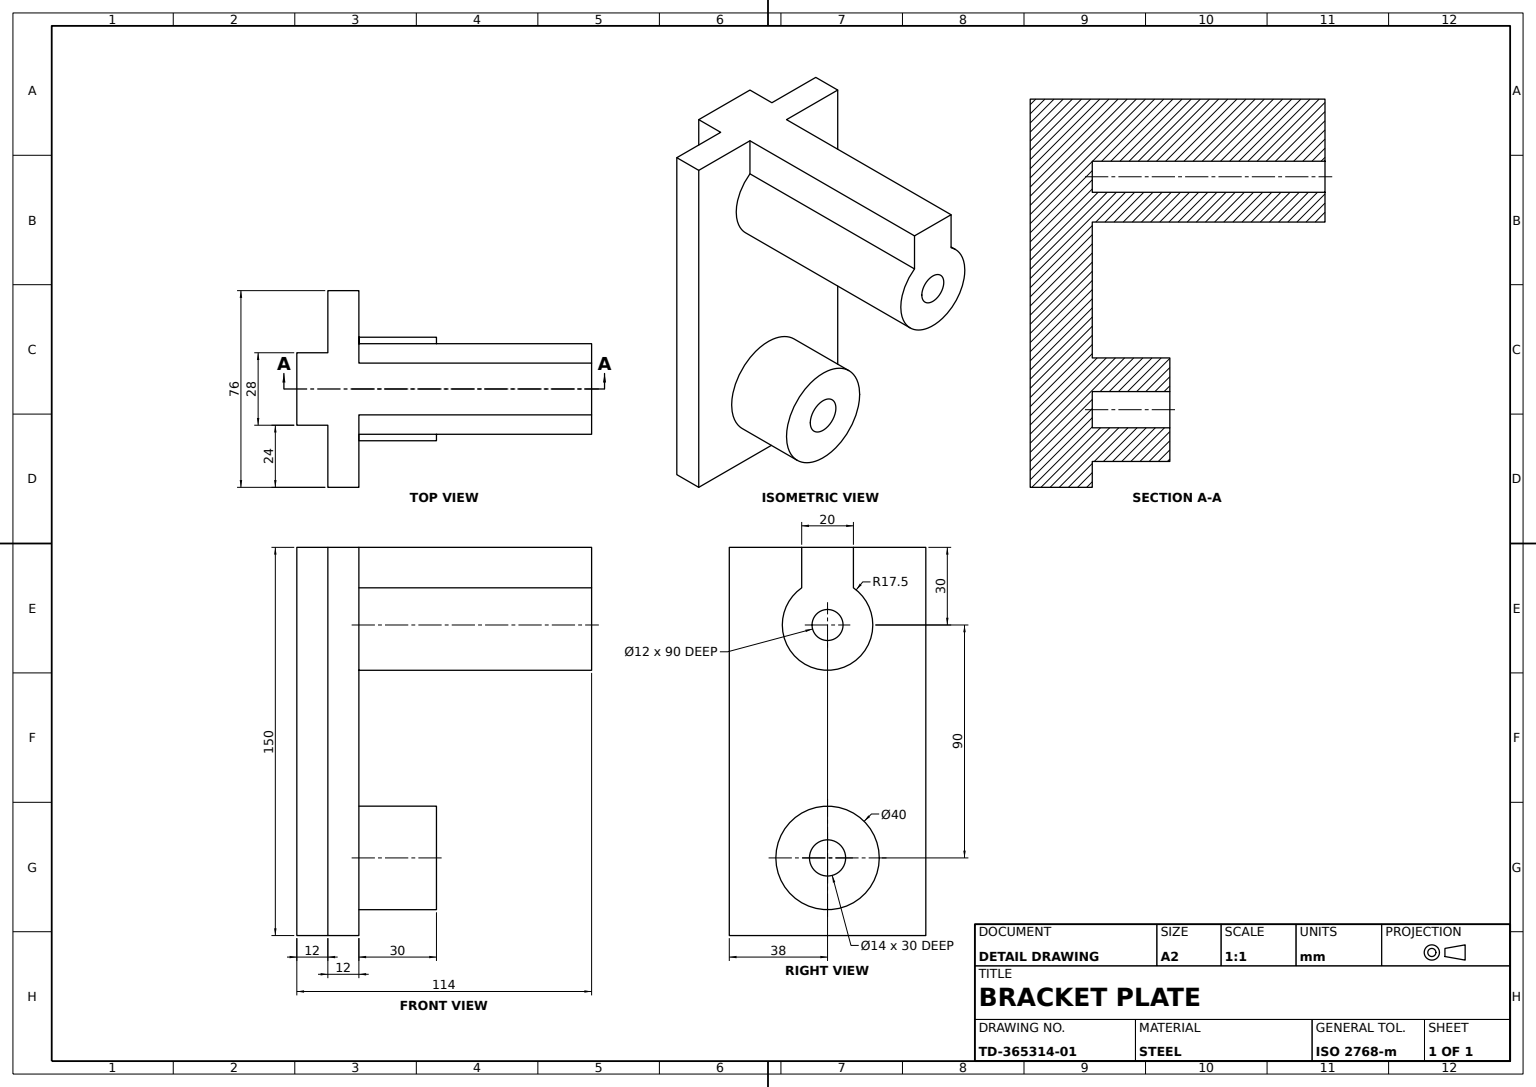
from build123d import *

# Parameters (mm, degrees)
BASE_PLATE_SKETCH_W           = 76
BASE_PLATE_SKETCH_H           = 150
BASE_PLATE_DEPTH              = 12
TOP_TAB_SKETCH_W              = 28
TOP_TAB_SKETCH_H              = 12
TOP_TAB_DEPTH                 = 150
LOWER_BUSHING_BOSS_SKETCH_R   = 20
LOWER_BUSHING_BOSS_SKETCH_R_2 = 7
LOWER_BUSHING_BOSS_DEPTH      = 30
UPPER_ARM_SKETCH_R            = 17.5
UPPER_ARM_SKETCH_R_2          = 6
UPPER_ARM_DEPTH               = 90
ARM_RIB_REACH                 = 187.332
ARM_RIB_END_RADIUS            = 17.5
ARM_RIB_SKETCH_W              = 20
ARM_RIB_SKETCH_H              = 90


with BuildPart() as part:
    # Base Plate Sketch → Base Plate (new body)
    with BuildSketch(Plane.XY):
        Rectangle(BASE_PLATE_SKETCH_W, BASE_PLATE_SKETCH_H)
    extrude(amount=BASE_PLATE_DEPTH)

    # Top Tab Sketch → Top Tab (add, through all)
    with BuildSketch(Plane.XZ.offset(75)):
        with Locations((0, -6)):
            Rectangle(TOP_TAB_SKETCH_W, TOP_TAB_SKETCH_H)
    extrude(amount=-TOP_TAB_DEPTH)

    # Lower Bushing Boss Sketch → Lower Bushing Boss (add)
    with BuildSketch(Plane.XY.offset(12)):
        with Locations(Location((0, -45, 0), (0, 0, 180))):
            Circle(LOWER_BUSHING_BOSS_SKETCH_R)
        with Locations((0, -45)):
            Circle(LOWER_BUSHING_BOSS_SKETCH_R_2, mode=Mode.SUBTRACT)
    extrude(amount=LOWER_BUSHING_BOSS_DEPTH)

    # Upper Arm Sketch → Upper Arm (add)
    with BuildSketch(Plane.XY.offset(12)):
        with Locations(Location((0, 45, 0), (0, 0, 180))):
            Circle(UPPER_ARM_SKETCH_R)
        with Locations(Location((0, 45, 0), (0, 0, 180))):
            Circle(UPPER_ARM_SKETCH_R_2, mode=Mode.SUBTRACT)
    extrude(amount=UPPER_ARM_DEPTH)

    # Arm Rib: up to this cylinder (the profile starts outside it)
    arm_rib_end = Plane(origin=(0, 45, 57), z_dir=(0, 0, -1)) * Cylinder(ARM_RIB_END_RADIUS, 410.664, mode=Mode.PRIVATE)
    # Arm Rib Sketch → Arm Rib (add, up to the surface)
    with BuildSketch(Plane(origin=(0, 75, 0), x_dir=(1, 0, 0), z_dir=(0, 1, 0)), mode=Mode.PRIVATE) as arm_rib_sk1:
        with Locations((0, -57)):
            Rectangle(ARM_RIB_SKETCH_W, ARM_RIB_SKETCH_H)
    arm_rib_tool1 = extrude(arm_rib_sk1.sketch, amount=-ARM_RIB_REACH, mode=Mode.PRIVATE) - arm_rib_end
    add(arm_rib_tool1.solids().sort_by_distance((0, 75, 57))[0])


solid = part.part
